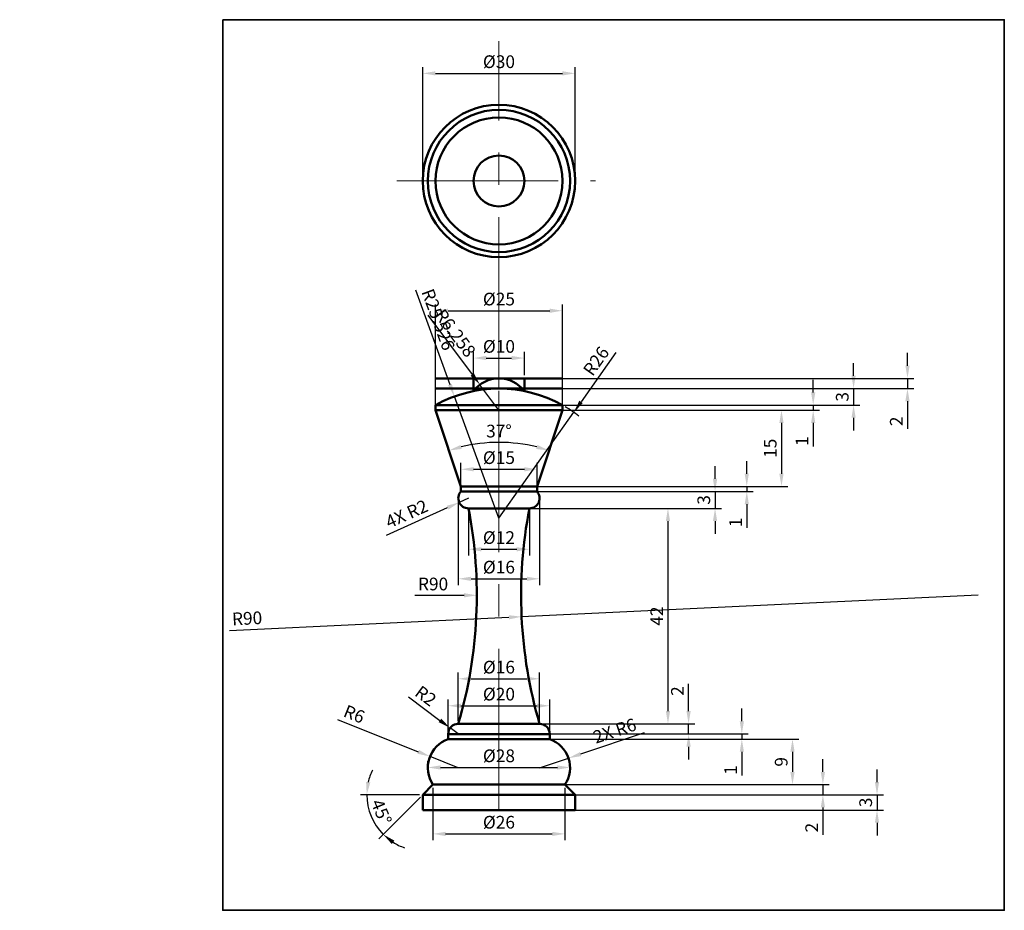
# Model space of a CAD drawing. Units: millimetres. Extents: x 388 to 582, y 164 to 339.
import ezdxf

# ---------------------------------------------------------------- set-up
doc = ezdxf.new("R2010")
doc.units = ezdxf.units.MM
doc.linetypes.add('CENTER', pattern=[50.8, 31.75, -6.35, 6.35, -6.35])
for name, color, linetype, lineweight in [('M-CNTR', 1, 'CENTER', 18), ('M-DIMS', 2, 'Continuous', 25), ('M-OUTL', 7, 'Continuous', 50), ('M-TTLB', 7, 'Continuous', 35)]:
    doc.layers.add(name, color=color, linetype=linetype, lineweight=lineweight)
doc.styles.get("Standard").update_dxf_attribs({"font": 'arial.ttf'})
doc.dimstyles.new('ISO-25', dxfattribs={"dimtxt": 2.5, "dimasz": 2.5, "dimexe": 1.25, "dimexo": 0.625, "dimtad": 1, "dimdec": 0, "dimtxsty": 'Standard', "dimcen": 2.5, "dimadec": 0, "dimazin": 0, "dimtfac": 1, "dimtdec": 0, "dimtmove": 0, "dimatfit": 3, "dimfxl": 1, "dimarcsym": 0})

# ---------------------------------------------------------------- blocks, each defined once
blk = doc.blocks.new('*D1')
at = {"layer": 'Defpoints', "color": 0, "transparency": 16777216}
for p in [(482.74, 268.57), (482.74, 266.57), (563.18, 266.57)]:
    blk.add_point(p, dxfattribs=at)
at = {"layer": 'M-DIMS', "color": 0, "lineweight": -2, "transparency": 16777216}
for p, q in [((563.18, 271.07), (563.18, 273.57)), ((483.37, 268.57), (564.43, 268.57)), ((563.18, 268.57), (563.18, 266.57)), ((483.37, 266.57), (564.43, 266.57)), ((563.18, 264.07), (563.18, 258.66))]:
    blk.add_line(p, q, dxfattribs=at)
at = {"layer": 'M-DIMS', "color": 0, "transparency": 16777216}
for points in [[(562.76, 271.07), (563.59, 271.07), (563.18, 268.57)], [(562.76, 264.07), (563.59, 264.07), (563.18, 266.57)]]:
    blk.add_solid(points, dxfattribs=at)
at = {"layer": 'M-DIMS', "color": 0, "transparency": 16777216, "insert": (561.3, 260.11), "char_height": 2.5, "attachment_point": 5, "rotation": 90}
blk.add_mtext('2', dxfattribs=at)
blk = doc.blocks.new('*D2')
at = {"layer": 'Defpoints', "color": 0, "transparency": 16777216}
for p in [(482.74, 266.57), (482.74, 263.3), (552.57, 263.3)]:
    blk.add_point(p, dxfattribs=at)
at = {"layer": 'M-DIMS', "color": 0, "lineweight": -2, "transparency": 16777216}
for p, q in [((552.57, 269.07), (552.57, 271.57)), ((483.37, 266.57), (553.82, 266.57)), ((552.57, 266.57), (552.57, 263.3)), ((483.37, 263.3), (553.82, 263.3)), ((552.57, 260.8), (552.57, 258.3))]:
    blk.add_line(p, q, dxfattribs=at)
at = {"layer": 'M-DIMS', "color": 0, "transparency": 16777216}
for points in [[(552.15, 269.07), (552.98, 269.07), (552.57, 266.57)], [(552.15, 260.8), (552.98, 260.8), (552.57, 263.3)]]:
    blk.add_solid(points, dxfattribs=at)
at = {"layer": 'M-DIMS', "color": 0, "transparency": 16777216, "insert": (550.66, 264.93), "char_height": 2.5, "attachment_point": 5, "rotation": 90}
blk.add_mtext('3', dxfattribs=at)
blk = doc.blocks.new('*D3')
at = {"layer": 'Defpoints', "color": 0, "transparency": 16777216}
for p in [(482.74, 263.3), (482.74, 262.3), (544.61, 262.3)]:
    blk.add_point(p, dxfattribs=at)
at = {"layer": 'M-DIMS', "color": 0, "lineweight": -2, "transparency": 16777216}
for p, q in [((544.61, 265.8), (544.61, 268.3)), ((483.37, 263.3), (545.86, 263.3)), ((483.37, 262.3), (545.86, 262.3)), ((544.61, 263.3), (544.61, 262.3)), ((544.61, 259.8), (544.61, 255.13))]:
    blk.add_line(p, q, dxfattribs=at)
at = {"layer": 'M-DIMS', "color": 0, "transparency": 16777216}
for points in [[(544.19, 265.8), (545.03, 265.8), (544.61, 263.3)], [(544.19, 259.8), (545.03, 259.8), (544.61, 262.3)]]:
    blk.add_solid(points, dxfattribs=at)
at = {"layer": 'M-DIMS', "color": 0, "transparency": 16777216, "insert": (542.73, 256.21), "char_height": 2.5, "attachment_point": 5, "rotation": 90}
blk.add_mtext('1', dxfattribs=at)
blk = doc.blocks.new('*D4')
at = {"layer": 'Defpoints', "color": 0, "transparency": 16777216}
for p in [(482.74, 262.3), (482.74, 247.3), (538.37, 247.3)]:
    blk.add_point(p, dxfattribs=at)
at = {"layer": 'M-DIMS', "color": 0, "lineweight": -2, "transparency": 16777216}
for p, q in [((483.37, 262.3), (539.62, 262.3)), ((538.37, 259.8), (538.37, 249.8)), ((483.37, 247.3), (539.62, 247.3))]:
    blk.add_line(p, q, dxfattribs=at)
at = {"layer": 'M-DIMS', "color": 0, "transparency": 16777216}
for points in [[(537.95, 259.8), (538.78, 259.8), (538.37, 262.3)], [(537.95, 249.8), (538.78, 249.8), (538.37, 247.3)]]:
    blk.add_solid(points, dxfattribs=at)
at = {"layer": 'M-DIMS', "color": 0, "transparency": 16777216, "insert": (536.47, 254.8), "char_height": 2.5, "attachment_point": 5, "rotation": 90}
blk.add_mtext('15', dxfattribs=at)
blk = doc.blocks.new('*D5')
at = {"layer": 'Defpoints', "color": 0, "transparency": 16777216}
for p in [(482.74, 247.3), (482.74, 246.3), (531.54, 246.3)]:
    blk.add_point(p, dxfattribs=at)
at = {"layer": 'M-DIMS', "color": 0, "lineweight": -2, "transparency": 16777216}
for p, q in [((531.54, 249.8), (531.54, 252.3)), ((483.37, 247.3), (532.79, 247.3)), ((483.37, 246.3), (532.79, 246.3)), ((531.54, 247.3), (531.54, 246.3)), ((531.54, 243.8), (531.54, 239.13))]:
    blk.add_line(p, q, dxfattribs=at)
at = {"layer": 'M-DIMS', "color": 0, "transparency": 16777216}
for points in [[(531.12, 249.8), (531.95, 249.8), (531.54, 247.3)], [(531.12, 243.8), (531.95, 243.8), (531.54, 246.3)]]:
    blk.add_solid(points, dxfattribs=at)
at = {"layer": 'M-DIMS', "color": 0, "transparency": 16777216, "insert": (529.66, 240.21), "char_height": 2.5, "attachment_point": 5, "rotation": 90}
blk.add_mtext('1', dxfattribs=at)
blk = doc.blocks.new('*D6')
at = {"layer": 'Defpoints', "color": 0, "transparency": 16777216}
for p in [(482.74, 246.3), (482.74, 242.98), (525.29, 242.98)]:
    blk.add_point(p, dxfattribs=at)
at = {"layer": 'M-DIMS', "color": 0, "lineweight": -2, "transparency": 16777216}
for p, q in [((525.29, 248.8), (525.29, 251.3)), ((483.37, 246.3), (526.54, 246.3)), ((525.29, 246.3), (525.29, 242.98)), ((483.37, 242.98), (526.54, 242.98)), ((525.29, 240.48), (525.29, 237.98))]:
    blk.add_line(p, q, dxfattribs=at)
at = {"layer": 'M-DIMS', "color": 0, "transparency": 16777216}
for points in [[(524.87, 248.8), (525.71, 248.8), (525.29, 246.3)], [(524.87, 240.48), (525.71, 240.48), (525.29, 242.98)]]:
    blk.add_solid(points, dxfattribs=at)
at = {"layer": 'M-DIMS', "color": 0, "transparency": 16777216, "insert": (523.39, 244.64), "char_height": 2.5, "attachment_point": 5, "rotation": 90}
blk.add_mtext('3', dxfattribs=at)
blk = doc.blocks.new('*D7')
at = {"layer": 'Defpoints', "color": 0, "transparency": 16777216}
for p in [(482.74, 242.98), (482.74, 200.55), (516.02, 200.55)]:
    blk.add_point(p, dxfattribs=at)
at = {"layer": 'M-DIMS', "color": 0, "lineweight": -2, "transparency": 16777216}
for p, q in [((483.37, 242.98), (517.27, 242.98)), ((516.02, 240.48), (516.02, 203.05)), ((483.37, 200.55), (517.27, 200.55))]:
    blk.add_line(p, q, dxfattribs=at)
at = {"layer": 'M-DIMS', "color": 0, "transparency": 16777216}
for points in [[(515.6, 240.48), (516.43, 240.48), (516.02, 242.98)], [(515.6, 203.05), (516.43, 203.05), (516.02, 200.55)]]:
    blk.add_solid(points, dxfattribs=at)
at = {"layer": 'M-DIMS', "color": 0, "transparency": 16777216, "insert": (514.14, 221.76), "char_height": 2.5, "attachment_point": 5, "rotation": 90}
blk.add_mtext('42', dxfattribs=at)
blk = doc.blocks.new('*D8')
at = {"layer": 'Defpoints', "color": 0, "transparency": 16777216}
for p in [(482.74, 200.55), (520.08, 200.55), (482.74, 198.55)]:
    blk.add_point(p, dxfattribs=at)
at = {"layer": 'M-DIMS', "color": 0, "lineweight": -2, "transparency": 16777216}
for p, q in [((520.08, 203.05), (520.08, 208.45)), ((483.37, 200.55), (521.33, 200.55)), ((520.08, 198.55), (520.08, 200.55)), ((483.37, 198.55), (521.33, 198.55)), ((520.08, 196.05), (520.08, 193.55))]:
    blk.add_line(p, q, dxfattribs=at)
at = {"layer": 'M-DIMS', "color": 0, "transparency": 16777216}
for points in [[(519.66, 203.05), (520.5, 203.05), (520.08, 200.55)], [(519.66, 196.05), (520.5, 196.05), (520.08, 198.55)]]:
    blk.add_solid(points, dxfattribs=at)
at = {"layer": 'M-DIMS', "color": 0, "transparency": 16777216, "insert": (518.2, 207), "char_height": 2.5, "attachment_point": 5, "rotation": 90}
blk.add_mtext('2', dxfattribs=at)
blk = doc.blocks.new('*D9')
at = {"layer": 'Defpoints', "color": 0, "transparency": 16777216}
for p in [(482.74, 198.55), (482.74, 197.55), (530.56, 197.55)]:
    blk.add_point(p, dxfattribs=at)
at = {"layer": 'M-DIMS', "color": 0, "lineweight": -2, "transparency": 16777216}
for p, q in [((530.56, 201.05), (530.56, 203.55)), ((483.37, 198.55), (531.81, 198.55)), ((530.56, 198.55), (530.56, 197.55)), ((483.37, 197.55), (531.81, 197.55)), ((530.56, 195.05), (530.56, 190.38))]:
    blk.add_line(p, q, dxfattribs=at)
at = {"layer": 'M-DIMS', "color": 0, "transparency": 16777216}
for points in [[(530.15, 201.05), (530.98, 201.05), (530.56, 198.55)], [(530.15, 195.05), (530.98, 195.05), (530.56, 197.55)]]:
    blk.add_solid(points, dxfattribs=at)
at = {"layer": 'M-DIMS', "color": 0, "transparency": 16777216, "insert": (528.68, 191.46), "char_height": 2.5, "attachment_point": 5, "rotation": 90}
blk.add_mtext('1', dxfattribs=at)
blk = doc.blocks.new('*D10')
at = {"layer": 'Defpoints', "color": 0, "transparency": 16777216}
for p in [(482.74, 197.55), (482.74, 188.58), (540.54, 188.58)]:
    blk.add_point(p, dxfattribs=at)
at = {"layer": 'M-DIMS', "color": 0, "lineweight": -2, "transparency": 16777216}
for p, q in [((483.37, 197.55), (541.79, 197.55)), ((540.54, 195.05), (540.54, 191.08)), ((483.37, 188.58), (541.79, 188.58))]:
    blk.add_line(p, q, dxfattribs=at)
at = {"layer": 'M-DIMS', "color": 0, "transparency": 16777216}
for points in [[(540.12, 195.05), (540.95, 195.05), (540.54, 197.55)], [(540.12, 191.08), (540.95, 191.08), (540.54, 188.58)]]:
    blk.add_solid(points, dxfattribs=at)
at = {"layer": 'M-DIMS', "color": 0, "transparency": 16777216, "insert": (538.64, 193.06), "char_height": 2.5, "attachment_point": 5, "rotation": 90}
blk.add_mtext('9', dxfattribs=at)
blk = doc.blocks.new('*D11')
at = {"layer": 'Defpoints', "color": 0, "transparency": 16777216}
for p in [(482.74, 188.58), (482.74, 186.58), (546.52, 186.58)]:
    blk.add_point(p, dxfattribs=at)
at = {"layer": 'M-DIMS', "color": 0, "lineweight": -2, "transparency": 16777216}
for p, q in [((546.52, 191.08), (546.52, 193.58)), ((483.37, 188.58), (547.77, 188.58)), ((546.52, 188.58), (546.52, 186.58)), ((483.37, 186.58), (547.77, 186.58)), ((546.52, 184.08), (546.52, 178.67))]:
    blk.add_line(p, q, dxfattribs=at)
at = {"layer": 'M-DIMS', "color": 0, "transparency": 16777216}
for points in [[(546.1, 191.08), (546.94, 191.08), (546.52, 188.58)], [(546.1, 184.08), (546.94, 184.08), (546.52, 186.58)]]:
    blk.add_solid(points, dxfattribs=at)
at = {"layer": 'M-DIMS', "color": 0, "transparency": 16777216, "insert": (544.64, 180.12), "char_height": 2.5, "attachment_point": 5, "rotation": 90}
blk.add_mtext('2', dxfattribs=at)
blk = doc.blocks.new('*D12')
at = {"layer": 'Defpoints', "color": 0, "transparency": 16777216}
for p in [(482.74, 186.58), (482.74, 183.58), (557.18, 183.58)]:
    blk.add_point(p, dxfattribs=at)
at = {"layer": 'M-DIMS', "color": 0, "lineweight": -2, "transparency": 16777216}
for p, q in [((557.18, 189.08), (557.18, 191.58)), ((483.37, 186.58), (558.43, 186.58)), ((557.18, 186.58), (557.18, 183.58)), ((483.37, 183.58), (558.43, 183.58)), ((557.18, 181.08), (557.18, 178.58))]:
    blk.add_line(p, q, dxfattribs=at)
at = {"layer": 'M-DIMS', "color": 0, "transparency": 16777216}
for points in [[(556.76, 189.08), (557.59, 189.08), (557.18, 186.58)], [(556.76, 181.08), (557.59, 181.08), (557.18, 183.58)]]:
    blk.add_solid(points, dxfattribs=at)
at = {"layer": 'M-DIMS', "color": 0, "transparency": 16777216, "insert": (555.27, 185.08), "char_height": 2.5, "attachment_point": 5, "rotation": 90}
blk.add_mtext('3', dxfattribs=at)
blk = doc.blocks.new('*D13')
at = {"layer": 'Defpoints', "color": 0, "transparency": 16777216}
for p in [(469.17, 194.12), (474.74, 191.89)]:
    blk.add_point(p, dxfattribs=at)
at = {"layer": 'M-DIMS', "color": 0, "lineweight": -2, "transparency": 16777216}
for p, q in [((450.97, 201.38), (466.85, 195.04)), ((474.74, 191.89), (469.17, 194.12))]:
    blk.add_line(p, q, dxfattribs=at)
at = {"layer": 'M-DIMS', "color": 0, "transparency": 16777216}
blk.add_solid([(467, 195.43), (466.69, 194.66), (469.17, 194.12)], dxfattribs=at)
at = {"layer": 'M-DIMS', "color": 0, "transparency": 16777216, "insert": (454.13, 202.17), "char_height": 2.5, "attachment_point": 5, "rotation": 338.2395}
blk.add_mtext('R6', dxfattribs=at)
blk = doc.blocks.new('*D14')
at = {"layer": 'Defpoints', "color": 0, "transparency": 16777216}
for p in [(496.74, 191.96), (468.74, 191.89), (496.74, 191.89)]:
    blk.add_point(p, dxfattribs=at)
at = {"layer": 'M-DIMS', "color": 0, "lineweight": -2, "transparency": 16777216}
for p, q in [((468.74, 192.52), (468.74, 193.21)), ((471.24, 191.96), (494.24, 191.96)), ((496.74, 192.52), (496.74, 193.21))]:
    blk.add_line(p, q, dxfattribs=at)
at = {"layer": 'M-DIMS', "color": 0, "transparency": 16777216}
for points in [[(471.24, 192.37), (471.24, 191.54), (468.74, 191.96)], [(494.24, 192.37), (494.24, 191.54), (496.74, 191.96)]]:
    blk.add_solid(points, dxfattribs=at)
at = {"layer": 'M-DIMS', "color": 0, "transparency": 16777216, "insert": (482.74, 193.93), "char_height": 2.5, "attachment_point": 5}
blk.add_mtext('%%C28', dxfattribs=at)
blk = doc.blocks.new('*D15')
at = {"layer": 'Defpoints', "color": 0, "transparency": 16777216}
for p in [(492.74, 204.11), (472.74, 198.55), (492.74, 198.55)]:
    blk.add_point(p, dxfattribs=at)
at = {"layer": 'M-DIMS', "color": 0, "lineweight": -2, "transparency": 16777216}
for p, q in [((472.74, 199.17), (472.74, 205.36)), ((475.24, 204.11), (490.24, 204.11)), ((492.74, 199.17), (492.74, 205.36))]:
    blk.add_line(p, q, dxfattribs=at)
at = {"layer": 'M-DIMS', "color": 0, "transparency": 16777216}
for points in [[(475.24, 204.52), (475.24, 203.69), (472.74, 204.11)], [(490.24, 204.52), (490.24, 203.69), (492.74, 204.11)]]:
    blk.add_solid(points, dxfattribs=at)
at = {"layer": 'M-DIMS', "color": 0, "transparency": 16777216, "insert": (482.74, 206.08), "char_height": 2.5, "attachment_point": 5}
blk.add_mtext('%%C20', dxfattribs=at)
blk = doc.blocks.new('*D16')
at = {"layer": 'Defpoints', "color": 0, "transparency": 16777216}
for p in [(490.74, 209.42), (474.74, 200.55), (490.74, 200.55)]:
    blk.add_point(p, dxfattribs=at)
at = {"layer": 'M-DIMS', "color": 0, "lineweight": -2, "transparency": 16777216}
for p, q in [((474.74, 201.17), (474.74, 210.67)), ((477.24, 209.42), (488.24, 209.42)), ((490.74, 201.17), (490.74, 210.67))]:
    blk.add_line(p, q, dxfattribs=at)
at = {"layer": 'M-DIMS', "color": 0, "transparency": 16777216}
for points in [[(477.24, 209.84), (477.24, 209), (474.74, 209.42)], [(488.24, 209.84), (488.24, 209), (490.74, 209.42)]]:
    blk.add_solid(points, dxfattribs=at)
at = {"layer": 'M-DIMS', "color": 0, "transparency": 16777216, "insert": (482.74, 211.39), "char_height": 2.5, "attachment_point": 5}
blk.add_mtext('%%C16', dxfattribs=at)
blk = doc.blocks.new('*D17')
at = {"layer": 'Defpoints', "color": 0, "transparency": 16777216}
for p in [(473.13, 199.74), (474.74, 198.55)]:
    blk.add_point(p, dxfattribs=at)
at = {"layer": 'M-DIMS', "color": 0, "lineweight": -2, "transparency": 16777216}
for p, q in [((464.9, 205.85), (471.13, 201.23)), ((474.74, 198.55), (473.13, 199.74))]:
    blk.add_line(p, q, dxfattribs=at)
at = {"layer": 'M-DIMS', "color": 0, "transparency": 16777216}
blk.add_solid([(471.37, 201.56), (470.88, 200.89), (473.13, 199.74)], dxfattribs=at)
at = {"layer": 'M-DIMS', "color": 0, "transparency": 16777216, "insert": (468.13, 205.79), "char_height": 2.5, "attachment_point": 5, "rotation": 323.4438}
blk.add_mtext('R2', dxfattribs=at)
blk = doc.blocks.new('*D18')
at = {"layer": 'Defpoints', "color": 0, "transparency": 16777216}
for p in [(388.38, 225.88), (478.38, 225.86)]:
    blk.add_point(p, dxfattribs=at)
at = {"layer": 'M-DIMS', "color": 0, "lineweight": -2, "transparency": 16777216}
blk.add_line((466.16, 225.86), (475.88, 225.86), dxfattribs=at)
at = {"layer": 'M-DIMS', "color": 0, "transparency": 16777216}
blk.add_solid([(475.88, 226.28), (475.88, 225.44), (478.38, 225.86)], dxfattribs=at)
at = {"layer": 'M-DIMS', "color": 0, "transparency": 16777216, "insert": (469.77, 227.76), "char_height": 2.5, "attachment_point": 5, "rotation": 359.9862}
blk.add_mtext('R90', dxfattribs=at)
blk = doc.blocks.new('*D19')
at = {"layer": 'Defpoints', "color": 0, "transparency": 16777216}
for p in [(476.74, 242.98), (488.74, 242.96), (488.74, 234.92)]:
    blk.add_point(p, dxfattribs=at)
at = {"layer": 'M-DIMS', "color": 0, "lineweight": -2, "transparency": 16777216}
for p, q in [((476.74, 242.35), (476.74, 233.67)), ((488.74, 242.34), (488.74, 233.67)), ((479.24, 234.92), (486.24, 234.92))]:
    blk.add_line(p, q, dxfattribs=at)
at = {"layer": 'M-DIMS', "color": 0, "transparency": 16777216}
for points in [[(479.24, 235.34), (479.24, 234.51), (476.74, 234.92)], [(486.24, 235.34), (486.24, 234.51), (488.74, 234.92)]]:
    blk.add_solid(points, dxfattribs=at)
at = {"layer": 'M-DIMS', "color": 0, "transparency": 16777216, "insert": (482.74, 236.9), "char_height": 2.5, "attachment_point": 5}
blk.add_mtext('%%C12', dxfattribs=at)
blk = doc.blocks.new('*D20')
at = {"layer": 'Defpoints', "color": 0, "transparency": 16777216}
for p in [(490.24, 250.67), (475.24, 246.3), (490.24, 246.3)]:
    blk.add_point(p, dxfattribs=at)
at = {"layer": 'M-DIMS', "color": 0, "lineweight": -2, "transparency": 16777216}
for p, q in [((475.24, 246.92), (475.24, 251.92)), ((477.74, 250.67), (487.74, 250.67)), ((490.24, 246.92), (490.24, 251.92))]:
    blk.add_line(p, q, dxfattribs=at)
at = {"layer": 'M-DIMS', "color": 0, "transparency": 16777216}
for points in [[(477.74, 251.09), (477.74, 250.26), (475.24, 250.67)], [(487.74, 251.09), (487.74, 250.26), (490.24, 250.67)]]:
    blk.add_solid(points, dxfattribs=at)
at = {"layer": 'M-DIMS', "color": 0, "transparency": 16777216, "insert": (482.74, 252.64), "char_height": 2.5, "attachment_point": 5}
blk.add_mtext('%%C15', dxfattribs=at)
blk = doc.blocks.new('*D21')
at = {"layer": 'Defpoints', "color": 0, "transparency": 16777216}
for p in [(474.74, 244.98), (490.74, 244.98), (490.74, 229.11)]:
    blk.add_point(p, dxfattribs=at)
at = {"layer": 'M-DIMS', "color": 0, "lineweight": -2, "transparency": 16777216}
for p, q in [((474.74, 244.35), (474.74, 227.86)), ((490.74, 244.35), (490.74, 227.86)), ((477.24, 229.11), (488.24, 229.11))]:
    blk.add_line(p, q, dxfattribs=at)
at = {"layer": 'M-DIMS', "color": 0, "transparency": 16777216}
for points in [[(477.24, 229.52), (477.24, 228.69), (474.74, 229.11)], [(488.24, 229.52), (488.24, 228.69), (490.74, 229.11)]]:
    blk.add_solid(points, dxfattribs=at)
at = {"layer": 'M-DIMS', "color": 0, "transparency": 16777216, "insert": (482.74, 231.08), "char_height": 2.5, "attachment_point": 5}
blk.add_mtext('%%C16', dxfattribs=at)
blk = doc.blocks.new('*D22')
at = {"layer": 'Defpoints', "color": 0, "transparency": 16777216}
for p in [(470.24, 262.3), (495.24, 262.3), (486.08, 255.79), (475.24, 247.3), (490.24, 247.3)]:
    blk.add_point(p, dxfattribs=at)
at = {"layer": 'M-DIMS', "color": 0, "lineweight": -2, "transparency": 16777216}
blk.add_arc((482.74, 224.8), 31.17, 76.1619, 103.8381, dxfattribs=at)
at = {"layer": 'M-DIMS', "color": 0, "transparency": 16777216}
for points in [[(475.4, 254.66), (475.17, 255.46), (472.88, 254.37)], [(490.31, 255.46), (490.08, 254.66), (492.6, 254.37)]]:
    blk.add_solid(points, dxfattribs=at)
at = {"layer": 'M-DIMS', "color": 0, "transparency": 16777216, "insert": (482.74, 257.87), "char_height": 2.5, "attachment_point": 5}
blk.add_mtext('37°', dxfattribs=at)
blk = doc.blocks.new('*D23')
at = {"layer": 'Defpoints', "color": 0, "transparency": 16777216}
for p in [(495.24, 281.89), (470.24, 262.3), (495.24, 262.3)]:
    blk.add_point(p, dxfattribs=at)
at = {"layer": 'M-DIMS', "color": 0, "lineweight": -2, "transparency": 16777216}
for p, q in [((470.24, 262.92), (470.24, 283.14)), ((495.24, 262.92), (495.24, 283.14)), ((472.74, 281.89), (492.74, 281.89))]:
    blk.add_line(p, q, dxfattribs=at)
at = {"layer": 'M-DIMS', "color": 0, "transparency": 16777216}
for points in [[(472.74, 282.3), (472.74, 281.47), (470.24, 281.89)], [(492.74, 282.3), (492.74, 281.47), (495.24, 281.89)]]:
    blk.add_solid(points, dxfattribs=at)
at = {"layer": 'M-DIMS', "color": 0, "transparency": 16777216, "insert": (482.74, 283.86), "char_height": 2.5, "attachment_point": 5}
blk.add_mtext('%%C25', dxfattribs=at)
blk = doc.blocks.new('*D24')
at = {"layer": 'Defpoints', "color": 0, "transparency": 16777216}
for p in [(469.74, 188.58), (467.74, 186.58), (467.74, 186.58), (497.74, 186.58), (457.08, 183.72)]:
    blk.add_point(p, dxfattribs=at)
at = {"layer": 'M-DIMS', "color": 0, "lineweight": -2, "transparency": 16777216}
for p, q in [((467.12, 186.58), (455.46, 186.58)), ((467.3, 186.14), (459.06, 177.89))]:
    blk.add_line(p, q, dxfattribs=at)
for start, end in [(153.9785, 166.9893), (180, 225), (238.0107, 251.0215)]:
    blk.add_arc((467.74, 186.58), 11.03, start, end, dxfattribs=at)
at = {"layer": 'M-DIMS', "color": 0, "transparency": 16777216}
for points in [[(457.41, 189.01), (456.58, 189.11), (456.71, 186.58)], [(461.64, 176.89), (462.16, 177.55), (459.94, 178.78)]]:
    blk.add_solid(points, dxfattribs=at)
at = {"layer": 'M-DIMS', "color": 0, "transparency": 16777216, "insert": (459.3, 183.08), "char_height": 2.5, "attachment_point": 5, "rotation": 292.5}
blk.add_mtext('45°', dxfattribs=at)
blk = doc.blocks.new('*D25')
at = {"layer": 'Defpoints', "color": 0, "transparency": 16777216}
for p in [(497.47, 261.89), (482.74, 241.04)]:
    blk.add_point(p, dxfattribs=at)
at = {"layer": 'M-DIMS', "color": 0, "lineweight": -2, "transparency": 16777216}
for p, q in [((505.77, 273.64), (498.91, 263.93)), ((482.74, 241.04), (497.47, 261.89))]:
    blk.add_line(p, q, dxfattribs=at)
blk.add_arc((482.74, 241.04), 25.53, 51.9527, 59.277, dxfattribs=at)
at = {"layer": 'M-DIMS', "color": 0, "transparency": 16777216}
blk.add_solid([(498.57, 264.17), (499.25, 263.69), (497.47, 261.89)], dxfattribs=at)
at = {"layer": 'M-DIMS', "color": 0, "transparency": 16777216, "insert": (502.13, 271.79), "char_height": 2.5, "attachment_point": 5, "rotation": 54.7584}
blk.add_mtext('R26', dxfattribs=at)
blk = doc.blocks.new('*D26')
at = {"layer": 'Defpoints', "color": 0, "transparency": 16777216}
for p in [(487.74, 272.57), (477.74, 268.57), (487.74, 268.57)]:
    blk.add_point(p, dxfattribs=at)
at = {"layer": 'M-DIMS', "color": 0, "lineweight": -2, "transparency": 16777216}
for p, q in [((477.74, 269.19), (477.74, 273.82)), ((487.74, 269.19), (487.74, 273.82)), ((480.24, 272.57), (485.24, 272.57))]:
    blk.add_line(p, q, dxfattribs=at)
at = {"layer": 'M-DIMS', "color": 0, "transparency": 16777216}
for points in [[(480.24, 272.99), (480.24, 272.16), (477.74, 272.57)], [(485.24, 272.99), (485.24, 272.16), (487.74, 272.57)]]:
    blk.add_solid(points, dxfattribs=at)
at = {"layer": 'M-DIMS', "color": 0, "transparency": 16777216, "insert": (482.74, 274.54), "char_height": 2.5, "attachment_point": 5}
blk.add_mtext('%%C10', dxfattribs=at)
blk = doc.blocks.new('*D27')
at = {"layer": 'Defpoints', "color": 0, "transparency": 16777216}
for p in [(497.74, 328.62), (467.74, 307.44), (497.74, 307.44)]:
    blk.add_point(p, dxfattribs=at)
at = {"layer": 'M-DIMS', "color": 0, "lineweight": -2, "transparency": 16777216}
for p, q in [((467.74, 308.07), (467.74, 329.87)), ((497.74, 308.07), (497.74, 329.87)), ((470.24, 328.62), (495.24, 328.62))]:
    blk.add_line(p, q, dxfattribs=at)
at = {"layer": 'M-DIMS', "color": 0, "transparency": 16777216}
for points in [[(470.24, 329.04), (470.24, 328.21), (467.74, 328.62)], [(495.24, 329.04), (495.24, 328.21), (497.74, 328.62)]]:
    blk.add_solid(points, dxfattribs=at)
at = {"layer": 'M-DIMS', "color": 0, "transparency": 16777216, "insert": (482.74, 330.6), "char_height": 2.5, "attachment_point": 5}
blk.add_mtext('%%C30', dxfattribs=at)
blk = doc.blocks.new('*D28')
at = {"layer": 'Defpoints', "color": 0, "transparency": 16777216}
for p in [(469.74, 188.58), (495.74, 188.58), (495.74, 178.88)]:
    blk.add_point(p, dxfattribs=at)
at = {"layer": 'M-DIMS', "color": 0, "lineweight": -2, "transparency": 16777216}
for p, q in [((469.74, 187.95), (469.74, 177.63)), ((495.74, 187.95), (495.74, 177.63)), ((472.24, 178.88), (493.24, 178.88))]:
    blk.add_line(p, q, dxfattribs=at)
at = {"layer": 'M-DIMS', "color": 0, "transparency": 16777216}
for points in [[(472.24, 179.29), (472.24, 178.46), (469.74, 178.88)], [(493.24, 179.29), (493.24, 178.46), (495.74, 178.88)]]:
    blk.add_solid(points, dxfattribs=at)
at = {"layer": 'M-DIMS', "color": 0, "transparency": 16777216, "insert": (482.74, 180.85), "char_height": 2.5, "attachment_point": 5}
blk.add_mtext('%%C26', dxfattribs=at)
blk = doc.blocks.new('*D29')
at = {"layer": 'Defpoints', "color": 0, "transparency": 16777216}
for p in [(577.1, 225.88), (487.2, 221.64)]:
    blk.add_point(p, dxfattribs=at)
at = {"layer": 'M-DIMS', "color": 0, "lineweight": -2, "transparency": 16777216}
for p, q in [((577.1, 225.88), (487.2, 221.64)), ((429.66, 218.93), (484.7, 221.53))]:
    blk.add_line(p, q, dxfattribs=at)
at = {"layer": 'M-DIMS', "color": 0, "transparency": 16777216}
blk.add_solid([(484.69, 221.94), (484.72, 221.11), (487.2, 221.64)], dxfattribs=at)
at = {"layer": 'M-DIMS', "color": 0, "transparency": 16777216, "insert": (433.17, 221), "char_height": 2.5, "attachment_point": 5, "rotation": 2.6986}
blk.add_mtext('R90', dxfattribs=at)
blk = doc.blocks.new('*D30')
at = {"layer": 'Defpoints', "color": 0, "transparency": 16777216}
for p in [(473.96, 265.01), (482.74, 241.04)]:
    blk.add_point(p, dxfattribs=at)
at = {"layer": 'M-DIMS', "color": 0, "lineweight": -2, "transparency": 16777216}
for p, q in [((466.28, 285.97), (473.1, 267.36)), ((482.74, 241.04), (473.96, 265.01))]:
    blk.add_line(p, q, dxfattribs=at)
at = {"layer": 'M-DIMS', "color": 0, "transparency": 16777216}
blk.add_solid([(473.49, 267.5), (472.71, 267.21), (473.96, 265.01)], dxfattribs=at)
at = {"layer": 'M-DIMS', "color": 0, "transparency": 16777216, "insert": (470.48, 280.04), "char_height": 2.5, "attachment_point": 5, "rotation": 290.1211}
blk.add_mtext('R25.526', dxfattribs=at)
blk = doc.blocks.new('*D31')
at = {"layer": 'Defpoints', "color": 0, "transparency": 16777216}
for p in [(478.99, 267.32), (482.74, 262.31)]:
    blk.add_point(p, dxfattribs=at)
at = {"layer": 'M-DIMS', "color": 0, "lineweight": -2, "transparency": 16777216}
for p, q in [((468.74, 280.99), (477.49, 269.32)), ((482.74, 262.31), (478.99, 267.32))]:
    blk.add_line(p, q, dxfattribs=at)
at = {"layer": 'M-DIMS', "color": 0, "transparency": 16777216}
blk.add_solid([(477.82, 269.57), (477.15, 269.07), (478.99, 267.32)], dxfattribs=at)
at = {"layer": 'M-DIMS', "color": 0, "transparency": 16777216, "insert": (473.89, 277.29), "char_height": 2.5, "attachment_point": 5, "rotation": 306.8548}
blk.add_mtext('R6.258', dxfattribs=at)
blk = doc.blocks.new('*D32')
at = {"layer": 'Defpoints', "color": 0, "transparency": 16777216}
for p in [(496.43, 193.79), (490.74, 191.89)]:
    blk.add_point(p, dxfattribs=at)
at = {"layer": 'M-DIMS', "color": 0, "lineweight": -2, "transparency": 16777216}
for p, q in [((511.31, 198.77), (498.8, 194.59)), ((490.74, 191.89), (496.43, 193.79))]:
    blk.add_line(p, q, dxfattribs=at)
at = {"layer": 'M-DIMS', "color": 0, "transparency": 16777216}
blk.add_solid([(498.67, 194.98), (498.93, 194.19), (496.43, 193.79)], dxfattribs=at)
at = {"layer": 'M-DIMS', "color": 0, "transparency": 16777216, "insert": (505.64, 198.88), "char_height": 2.5, "attachment_point": 5, "rotation": 18.4902}
blk.add_mtext('2X R6', dxfattribs=at)
blk = doc.blocks.new('*D33')
at = {"layer": 'Defpoints', "color": 0, "transparency": 16777216}
for p in [(476.74, 244.98), (474.92, 244.15)]:
    blk.add_point(p, dxfattribs=at)
at = {"layer": 'M-DIMS', "color": 0, "lineweight": -2, "transparency": 16777216}
for p, q in [((476.74, 244.98), (474.92, 244.15)), ((460.59, 237.68), (472.64, 243.12))]:
    blk.add_line(p, q, dxfattribs=at)
at = {"layer": 'M-DIMS', "color": 0, "transparency": 16777216}
blk.add_solid([(472.47, 243.5), (472.81, 242.74), (474.92, 244.15)], dxfattribs=at)
at = {"layer": 'M-DIMS', "color": 0, "transparency": 16777216, "insert": (464.7, 241.6), "char_height": 2.5, "attachment_point": 5, "rotation": 24.3146}
blk.add_mtext('4X R2', dxfattribs=at)

msp = doc.modelspace()

# ---------------------------------------------------------------- linework, layer by layer
at = {"layer": 'M-CNTR'}
for p, q in [((482.7411, 268.5675), (482.7411, 334.9406)), ((462.6587, 307.4406), (501.7248, 307.4406)), ((482.7411, 267.1418), (482.7411, 268.5675)), ((482.7411, 266.5675), (482.7411, 267.1418)), ((482.7411, 183.5775), (482.7411, 266.5675))]:
    msp.add_line(p, q, dxfattribs=at)
at = {"layer": 'M-OUTL'}
for p, q in [((482.7411, 268.5675), (470.2411, 268.5675)), ((477.7411, 266.073), (477.7411, 268.5675)), ((482.7411, 268.5675), (495.2411, 268.5675)), ((487.7411, 266.073), (487.7411, 268.5675)), ((482.7411, 266.5675), (470.2411, 266.5675)), ((482.7411, 266.5675), (495.2411, 266.5675)), ((482.7411, 263.2975), (470.2411, 263.2975)), ((470.2411, 262.2975), (470.2411, 263.2975)), ((482.7411, 262.2975), (470.2411, 262.2975)), ((470.2411, 262.2975), (475.2411, 247.2975)), ((482.7411, 263.2975), (495.2411, 263.2975)), ((482.7411, 262.2975), (495.2411, 262.2975)), ((490.2411, 247.2975), (495.2411, 262.2975)), ((495.2411, 262.2975), (495.2411, 263.2975)), ((482.7411, 247.2975), (475.2411, 247.2975)), ((475.2411, 246.2975), (475.2411, 247.2975)), ((482.7411, 246.2975), (475.2411, 246.2975)), ((482.7411, 247.2975), (490.2411, 247.2975)), ((482.7411, 246.2975), (490.2411, 246.2975)), ((490.2411, 247.2975), (490.2411, 246.2975)), ((482.7411, 242.9775), (476.7411, 242.9775)), ((482.7411, 242.9775), (488.7411, 242.9775)), ((482.7411, 200.5475), (474.7411, 200.5475)), ((482.7411, 200.5475), (490.7411, 200.5475)), ((482.7411, 198.5475), (472.7411, 198.5475)), ((472.7411, 197.5475), (472.7411, 198.5475)), ((482.7411, 198.5475), (492.7411, 198.5475)), ((492.7411, 197.5475), (492.7411, 198.5475)), ((482.7411, 197.5475), (472.7411, 197.5475)), ((482.7411, 197.5475), (492.7411, 197.5475)), ((467.7411, 186.5775), (469.7411, 188.5775)), ((482.7411, 188.5775), (469.7411, 188.5775)), ((482.7411, 188.5775), (495.7411, 188.5775)), ((495.7411, 188.5775), (497.7411, 186.5775)), ((497.7411, 186.5775), (467.7411, 186.5775)), ((467.7411, 186.5775), (467.7411, 183.5775)), ((497.7411, 183.5775), (497.7411, 186.5775)), ((467.7411, 183.5775), (497.7411, 183.5775))]:
    msp.add_line(p, q, dxfattribs=at)
for radius in [15, 14, 12.5, 5]:
    msp.add_circle((482.7411, 307.4406), radius, dxfattribs=at)
for centre, radius, start, end in [((482.7411, 262.3091), 6.2583, 36.971555, 143.028445), ((482.7411, 241.0411), 25.5264, 60.679898, 119.320102), ((476.7436, 244.9775), 2, 138.700066, 269.927527), ((488.7386, 244.9775), 2, 270.072473, 41.299934), ((388.38, 225.8804), 90, 343.651647, 10.950907), ((577.1022, 225.8804), 90, 169.049093, 196.348353), ((474.7411, 198.5475), 2, 90, 180), ((490.7411, 198.5475), 2, 0, 90), ((474.743, 191.8913), 6, 109.490144, 213.525022), ((490.7392, 191.8913), 6, 326.474978, 70.509856)]:
    msp.add_arc(centre, radius, start, end, dxfattribs=at)
at = {"layer": 'M-TTLB'}
msp.add_lwpolyline([(428.3759, 339.1918), (582.2405, 339.1918), (582.2405, 163.8343), (428.3759, 163.8343)], close=True, dxfattribs=at)

# ---------------------------------------------------------------- dimensions: what is measured, and where the dimension line sits
at = {"layer": 'M-DIMS'}
for base, p1, p2, picture, middle in [((497.7411, 328.6243), (467.7411, 307.4406), (497.7411, 307.4406), '*D27', (482.7411, 330.5957)), ((495.2411, 281.8857), (470.2411, 262.2975), (495.2411, 262.2975), '*D23', (482.7411, 283.857)), ((487.7411, 272.5725), (477.7411, 268.5675), (487.7411, 268.5675), '*D26', (482.7411, 274.5439)), ((490.2411, 250.6729), (475.2411, 246.2975), (490.2411, 246.2975), '*D20', (482.7411, 252.6442)), ((490.7386, 229.1082), (474.7436, 244.9775), (490.7386, 244.9775), '*D21', (482.7411, 231.0795)), ((488.7382, 234.9243), (476.7411, 242.9775), (488.7382, 242.9623), '*D19', (482.7396, 236.8956)), ((490.7411, 209.4208), (474.7411, 200.5475), (490.7411, 200.5475), '*D16', (482.7411, 211.3922)), ((492.7411, 204.1054), (472.7411, 198.5475), (492.7411, 198.5475), '*D15', (482.7411, 206.0768)), ((496.7392, 191.9573), (468.743, 191.8913), (496.7392, 191.8913), '*D14', (482.7411, 193.9286)), ((495.7411, 178.8768), (469.7411, 188.5775), (495.7411, 188.5775), '*D28', (482.7411, 180.8482))]:
    dim = msp.add_linear_dim(base=base, p1=p1, p2=p2, text='%%C<>', dimstyle='ISO-25', override={"dimclrd": 0, "dimclre": 0, "dimclrt": 0}, dxfattribs=at)
    dim.commit()
    dim.dimension.update_dxf_attribs({"geometry": picture, "text_midpoint": middle})
for center, mpoint, override, picture, middle in [((482.7411, 241.0411), (473.9599, 265.0096), {"dimdec": 3, "dimlfac": 1, "dimrnd": 0, "dimzin": 0, "dimdsep": 46, "dimlunit": 2}, '*D30', (468.6911, 279.3907)), ((482.7411, 241.0411), (497.4705, 261.8892), {"dimclrd": 0, "dimclre": 0, "dimclrt": 0}, '*D25', (503.6873, 270.6884)), ((388.38, 225.8804), (478.38, 225.8588), {"dimclrd": 0, "dimclre": 0, "dimclrt": 0}, '*D18', (469.7724, 225.8609)), ((577.1022, 225.8804), (487.202, 221.643), {"dimdec": 0, "dimlfac": 1, "dimrnd": 0, "dimzin": 0, "dimdsep": 46, "dimlunit": 2}, '*D29', (433.2619, 219.1006)), ((474.743, 191.8913), (469.1705, 194.1157), {"dimclrd": 0, "dimclre": 0, "dimclrt": 0}, '*D13', (453.4219, 200.402))]:
    dim = msp.add_radius_dim(center=center, mpoint=mpoint, dimstyle='ISO-25', override=override, dxfattribs=at)
    dim.commit()
    dim.dimension.update_dxf_attribs({"geometry": picture, "text_midpoint": middle, "dimtype": 164})
for center, mpoint, override, picture, middle in [((482.7411, 262.3091), (478.9874, 267.3168), {"dimdec": 3, "dimlfac": 1, "dimrnd": 0, "dimzin": 0, "dimdsep": 46, "dimlunit": 2}, '*D31', (473.886, 277.2926)), ((474.7411, 198.5475), (473.1345, 199.7387), {"dimclrd": 0, "dimclre": 0, "dimclrt": 0}, '*D17', (468.1271, 205.7922))]:
    dim = msp.add_radius_dim(center=center, mpoint=mpoint, dimstyle='ISO-25', override=override, dxfattribs=at)
    dim.commit()
    dim.dimension.update_dxf_attribs({"geometry": picture, "text_midpoint": middle})
for base, p1, p2, picture, middle in [((563.1775, 266.5675), (482.7411, 268.5675), (482.7411, 266.5675), '*D1', (561.2974, 260.1146)), ((552.5668, 263.2975), (482.7411, 266.5675), (482.7411, 263.2975), '*D2', (550.6645, 264.9325)), ((544.6088, 262.2975), (482.7411, 263.2975), (482.7411, 262.2975), '*D3', (542.7287, 256.2121)), ((531.5355, 246.2975), (482.7411, 247.2975), (482.7411, 246.2975), '*D5', (529.6554, 240.2121)), ((525.2906, 242.9775), (482.7411, 246.2975), (482.7411, 242.9775), '*D6', (523.3883, 244.6375)), ((516.0172, 200.5475), (482.7411, 242.9775), (482.7411, 200.5475), '*D7', (514.1371, 221.7625)), ((520.0796, 200.5475), (482.7411, 198.5475), (482.7411, 200.5475), '*D8', (518.1995, 207.0004)), ((530.5626, 197.5475), (482.7411, 198.5475), (482.7411, 197.5475), '*D9', (528.6825, 191.4621)), ((540.5371, 188.5775), (482.7411, 197.5475), (482.7411, 188.5775), '*D10', (538.6357, 193.0625)), ((546.5202, 186.5775), (482.7411, 188.5775), (482.7411, 186.5775), '*D11', (544.6401, 180.1246)), ((557.1752, 183.5775), (482.7411, 186.5775), (482.7411, 183.5775), '*D12', (555.2729, 185.0775))]:
    dim = msp.add_linear_dim(base=base, p1=p1, p2=p2, angle=90, dimstyle='ISO-25', override={"dimclrd": 0, "dimclre": 0, "dimclrt": 0}, dxfattribs=at)
    dim.commit()
    dim.dimension.update_dxf_attribs({"geometry": picture, "text_midpoint": middle})
for base, line1, line2, picture, middle in [((486.0776, 255.7874), ((490.2411, 247.2975), (495.2411, 262.2975)), ((470.2411, 262.2975), (475.2411, 247.2975)), '*D22', (482.7411, 257.8688)), ((457.084, 183.7219), ((497.7411, 186.5775), (467.7411, 186.5775)), ((467.7411, 186.5775), (469.7411, 188.5775)), '*D24', (459.2999, 183.081))]:
    dim = msp.add_angular_dim_2l(base=base, line1=line1, line2=line2, dimstyle='ISO-25', override={"dimclrd": 0, "dimclre": 0, "dimclrt": 0}, dxfattribs=at)
    dim.commit()
    dim.dimension.update_dxf_attribs({"geometry": picture, "text_midpoint": middle})
dim = msp.add_linear_dim(base=(538.3672, 247.2975), p1=(482.7411, 262.2975), p2=(482.7411, 247.2975), angle=90, dimstyle='ISO-25', override={"dimclrd": 0, "dimclre": 0, "dimclrt": 0}, dxfattribs=at)
dim.commit()
dim.dimension.update_dxf_attribs({"geometry": '*D4', "text_midpoint": (538.3672, 254.7975), "dimtype": 160})
for center, mpoint, text, picture, middle in [((476.7436, 244.9775), (474.921, 244.154), '4X <>', '*D33', (464.7018, 241.6008)), ((490.7392, 191.8913), (496.4295, 193.7942), '2X <>', '*D32', (505.6394, 198.8789))]:
    dim = msp.add_radius_dim(center=center, mpoint=mpoint, text=text, dimstyle='ISO-25', override={"dimdec": 0, "dimlfac": 1, "dimrnd": 0, "dimzin": 0, "dimdsep": 46, "dimlunit": 2}, dxfattribs=at)
    dim.commit()
    dim.dimension.update_dxf_attribs({"geometry": picture, "text_midpoint": middle})

doc.saveas('drawing.dxf')
